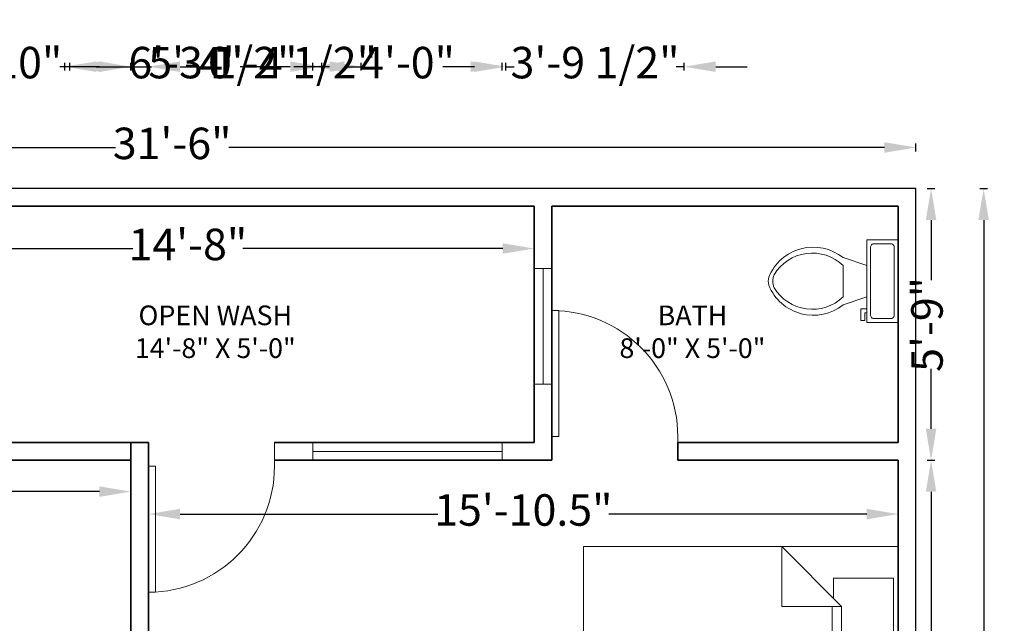
# Model space of a CAD drawing. Units: inches. Extents: x 2174 to 2692, y 577 to 1264.
# Tile 5 of 5: x 2442 to 2692, y 1110 to 1263. Entities that reach past the tile are written whole.
import ezdxf

# ---------------------------------------------------------------- set-up
doc = ezdxf.new("R2010")
doc.units = ezdxf.units.IN
for name, color, linetype, lineweight in [('A-ANNO-DIMS', 2, 'Continuous', 13), ('A-AREA-IDEN', 7, 'Continuous', 18), ('A-DOOR', 3, 'Continuous', 18), ('A-FLOR-FIXT', 9, 'Continuous', 18), ('A-FURN', 8, 'Continuous', 18), ('A-GLAZ', 4, 'Continuous', 18), ('A-WALL', 7, 'Continuous', 35), ('C-PROP', 7, 'Continuous', 25)]:
    doc.layers.add(name, color=color, linetype=linetype, lineweight=lineweight)
doc.styles.get("Standard").update_dxf_attribs({"font": 'arial.ttf'})
doc.dimstyles.new('ISO-25', dxfattribs={"dimtxt": 8, "dimasz": 8, "dimexe": 1, "dimexo": 1, "dimtad": 0, "dimdec": 1, "dimlunit": 3, "dimtxsty": 'Standard', "dimcen": 2.5, "dimclrd": 1, "dimclre": 1, "dimclrt": 1, "dimadec": 0, "dimazin": 0, "dimtfac": 1, "dimtdec": 1, "dimtmove": 0, "dimatfit": 3, "dimfxl": 1, "dimfxlon": 1, "dimarcsym": 0})

# ---------------------------------------------------------------- blocks, each defined once
blk = doc.blocks.new('Bed - Queen')
for p, q in [((0, -80.00003), (0, 0)), ((0, 0), (59.99999, 0)), ((59.99999, 0), (59.99999, -80.00003)), ((7.99999, -1.2), (28.79998, -1.2)), ((7.99999, -14.4), (7.99999, -1.2)), ((28.79998, -1.2), (28.79998, -14.4)), ((31.19999, -1.2), (51.99999, -1.2)), ((31.19999, -14.4), (31.19999, -1.2)), ((51.99999, -1.2), (51.99999, -16.4)), ((0, -14.4), (44.8, -14.4)), ((59.99999, -29.6), (44.8, -14.4)), ((44.8, -14.4), (44.8, -29.6)), ((44.8, -16.8), (0, -16.8)), ((51.99999, -16.4), (46.79936, -16.4)), ((44.8, -29.6), (59.99999, -29.6)), ((59.99999, -80.00003), (0, -80.00003))]:
    blk.add_line(p, q)
blk = doc.blocks.new('Toilet - top')
for p, q in [((9.5, -6), (9.5, -2)), ((-10, -8.5), (-8, -8.5)), ((-10, -9.5), (-10, -8.5)), ((-7, -9.5), (-10, -9.5)), ((-8, -8.5), (-8, -8)), ((-7, -8), (-7, -9.5)), ((-4, -8), (-6, -14)), ((4, -8), (6, -14)), ((4, -14), (-4, -14))]:
    blk.add_line(p, q)
blk.add_lwpolyline([(10.5, -8), (10.5, 0), (-10.5, 0), (-10.5, -8)], close=True)
for points in [[(-9.5, -2), (-9.5, -6)], [(8.5, -1), (-8.5, -1)], [(-8.5, -7), (8.5, -7)]]:
    blk.add_lwpolyline(points)
for centre, radius, start, end in [((-8.62, -1.88), 0.884, 81.8699, 188.1301), ((8.62, -1.88), 0.884, 351.8699, 98.1301), ((-8.62, -6.12), 0.884, 171.8699, 278.1301), ((8.62, -6.12), 0.884, 261.8699, 8.1301), ((3.52, -21.58), 12.17, 141.4691, 247.9714), ((4.2, -21.82), 11.33, 136.3677, 238.9468), ((-3.52, -21.58), 12.17, 292.0284, 38.5307), ((-4.2, -21.82), 11.33, 301.053, 43.6321), ((0, -27.88), 4, 245.7318, 294.2682), ((0, -29), 4, 254.8605, 285.1395)]:
    blk.add_arc(centre, radius, start, end)
blk = doc.blocks.new('*D9')
at = {"layer": 'A-ANNO-DIMS', "color": 0, "lineweight": -2, "transparency": 16777216}
for p, q in [((2396.95, 1206.12), (2396.95, 1204.12)), ((2572.95, 1206.12), (2572.95, 1204.12)), ((2404.95, 1205.12), (2470.96, 1205.12)), ((2564.95, 1205.12), (2498.94, 1205.12))]:
    blk.add_line(p, q, dxfattribs=at)
at = {"layer": 'A-ANNO-DIMS', "color": 0, "transparency": 16777216}
for points in [[(2404.95, 1206.46), (2404.95, 1203.79), (2396.95, 1205.12)], [(2564.95, 1206.46), (2564.95, 1203.79), (2572.95, 1205.12)]]:
    blk.add_solid(points, dxfattribs=at)
at = {"layer": 'Defpoints', "color": 0, "transparency": 16777216}
for p in [(2396.95, 1215.85), (2572.95, 1215.85), (2396.95, 1205.12)]:
    blk.add_point(p, dxfattribs=at)
at = {"layer": 'A-ANNO-DIMS', "color": 0, "transparency": 16777216, "insert": (2484.95, 1205.12), "char_height": 8, "attachment_point": 5}
blk.add_mtext('14\'-8"', dxfattribs=at)
blk = doc.blocks.new('*D10')
at = {"layer": 'A-ANNO-DIMS', "color": 0, "lineweight": -2, "transparency": 16777216}
for p, q in [((2665.45, 1137.68), (2665.45, 1138.68)), ((2474.95, 1137.68), (2474.95, 1136.68)), ((2482.95, 1137.68), (2548.45, 1137.68)), ((2657.45, 1137.68), (2591.96, 1137.68))]:
    blk.add_line(p, q, dxfattribs=at)
at = {"layer": 'A-ANNO-DIMS', "color": 0, "transparency": 16777216}
for points in [[(2482.95, 1139.02), (2482.95, 1136.35), (2474.95, 1137.68)], [(2657.45, 1139.02), (2657.45, 1136.35), (2665.45, 1137.68)]]:
    blk.add_solid(points, dxfattribs=at)
at = {"layer": 'Defpoints', "color": 0, "transparency": 16777216}
for p in [(2474.95, 1137.68), (2665.45, 1137.68), (2665.45, 1137.68)]:
    blk.add_point(p, dxfattribs=at)
at = {"layer": 'A-ANNO-DIMS', "color": 0, "transparency": 16777216, "insert": (2570.2, 1137.68), "char_height": 8, "attachment_point": 5}
blk.add_mtext('15\'-10.5"', dxfattribs=at)
blk = doc.blocks.new('*D11')
at = {"layer": 'A-ANNO-DIMS', "color": 0, "lineweight": -2, "transparency": 16777216}
for p, q in [((2296.45, 1144.39), (2296.45, 1142.39)), ((2470.45, 1144.39), (2470.45, 1142.39)), ((2304.45, 1143.39), (2369.46, 1143.39)), ((2462.45, 1143.39), (2397.44, 1143.39))]:
    blk.add_line(p, q, dxfattribs=at)
at = {"layer": 'A-ANNO-DIMS', "color": 0, "transparency": 16777216}
for points in [[(2304.45, 1144.72), (2304.45, 1142.05), (2296.45, 1143.39)], [(2462.45, 1144.72), (2462.45, 1142.05), (2470.45, 1143.39)]]:
    blk.add_solid(points, dxfattribs=at)
at = {"layer": 'Defpoints', "color": 0, "transparency": 16777216}
for p in [(2296.45, 1151.35), (2470.45, 1151.35), (2470.45, 1143.39)]:
    blk.add_point(p, dxfattribs=at)
at = {"layer": 'A-ANNO-DIMS', "color": 0, "transparency": 16777216, "insert": (2383.45, 1143.39), "char_height": 8, "attachment_point": 5}
blk.add_mtext('14\'-6"', dxfattribs=at)
blk = doc.blocks.new('*U23')
for p, q in [((0, 0), (0, 6)), ((32, 0), (32, 6))]:
    blk.add_line(p, q)
blk.add_lwpolyline([(0, 0), (0, -32), (1.75, -32), (1.75, 0)], close=True)
blk.add_arc((0, 0), 32, 270, 0)
blk = doc.blocks.new('*U22')
for p, q in [((0, 0), (0, -6)), ((32, 0), (32, -6))]:
    blk.add_line(p, q)
blk.add_lwpolyline([(0, 0), (0, 32), (1.75, 32), (1.75, 0)], close=True)
blk.add_arc((0, 0), 32, 0, 90)
blk = doc.blocks.new('*D28')
at = {"layer": 'A-ANNO-DIMS', "color": 0, "lineweight": -2, "transparency": 16777216}
for p, q in [((2291.95, 1229.78), (2291.95, 1231.78)), ((2669.95, 1229.78), (2669.95, 1231.78)), ((2299.95, 1230.78), (2466.59, 1230.78)), ((2661.95, 1230.78), (2495.32, 1230.78))]:
    blk.add_line(p, q, dxfattribs=at)
at = {"layer": 'A-ANNO-DIMS', "color": 0, "transparency": 16777216}
for points in [[(2299.95, 1232.11), (2299.95, 1229.44), (2291.95, 1230.78)], [(2661.95, 1232.11), (2661.95, 1229.44), (2669.95, 1230.78)]]:
    blk.add_solid(points, dxfattribs=at)
at = {"layer": 'Defpoints', "color": 0, "transparency": 16777216}
for p in [(2669.95, 1230.78), (2291.95, 1220.35), (2669.95, 1220.35)]:
    blk.add_point(p, dxfattribs=at)
at = {"layer": 'A-ANNO-DIMS', "color": 0, "transparency": 16777216, "insert": (2480.95, 1230.78), "char_height": 8, "attachment_point": 5}
blk.add_mtext('31\'-6"', dxfattribs=at)
blk = doc.blocks.new('*D35')
at = {"layer": 'A-ANNO-DIMS', "color": 0, "lineweight": -2, "transparency": 16777216}
for p, q in [((2672.81, 1220.35), (2674.81, 1220.35)), ((2673.81, 1212.35), (2673.81, 1197.11)), ((2673.81, 1159.35), (2673.81, 1174.59)), ((2672.81, 1151.35), (2674.81, 1151.35))]:
    blk.add_line(p, q, dxfattribs=at)
at = {"layer": 'A-ANNO-DIMS', "color": 0, "transparency": 16777216}
for points in [[(2672.48, 1212.35), (2675.15, 1212.35), (2673.81, 1220.35)], [(2672.48, 1159.35), (2675.15, 1159.35), (2673.81, 1151.35)]]:
    blk.add_solid(points, dxfattribs=at)
at = {"layer": 'Defpoints', "color": 0, "transparency": 16777216}
for p in [(2669.95, 1220.35), (2665.45, 1151.35), (2673.81, 1151.35)]:
    blk.add_point(p, dxfattribs=at)
at = {"layer": 'A-ANNO-DIMS', "color": 0, "transparency": 16777216, "insert": (2673.81, 1185.85), "char_height": 8, "attachment_point": 5, "rotation": 90}
blk.add_mtext('5\'-9"', dxfattribs=at)
blk = doc.blocks.new('*D36')
at = {"layer": 'A-ANNO-DIMS', "color": 0, "lineweight": -2, "transparency": 16777216}
for p, q in [((2672.81, 1151.35), (2674.81, 1151.35)), ((2673.81, 1143.35), (2673.81, 1101.75)), ((2673.81, 1022.85), (2673.81, 1064.45)), ((2672.81, 1014.85), (2674.81, 1014.85))]:
    blk.add_line(p, q, dxfattribs=at)
at = {"layer": 'A-ANNO-DIMS', "color": 0, "transparency": 16777216}
for points in [[(2672.48, 1143.35), (2675.15, 1143.35), (2673.81, 1151.35)], [(2672.48, 1022.85), (2675.15, 1022.85), (2673.81, 1014.85)]]:
    blk.add_solid(points, dxfattribs=at)
at = {"layer": 'Defpoints', "color": 0, "transparency": 16777216}
for p in [(2665.45, 1151.35), (2665.45, 1014.85), (2673.81, 1014.85)]:
    blk.add_point(p, dxfattribs=at)
at = {"layer": 'A-ANNO-DIMS', "color": 0, "transparency": 16777216, "insert": (2673.81, 1083.1), "char_height": 8, "attachment_point": 5, "rotation": 90}
blk.add_mtext('11\'-4.5"', dxfattribs=at)
blk = doc.blocks.new('*D42')
at = {"layer": 'A-ANNO-DIMS', "color": 0, "lineweight": -2, "transparency": 16777216}
for p, q in [((2686.18, 1220.35), (2688.18, 1220.35)), ((2687.18, 1212.35), (2687.18, 927.77)), ((2687.18, 628.35), (2687.18, 912.94)), ((2686.18, 620.35), (2688.18, 620.35))]:
    blk.add_line(p, q, dxfattribs=at)
at = {"layer": 'A-ANNO-DIMS', "color": 0, "transparency": 16777216}
for points in [[(2685.84, 1212.35), (2688.51, 1212.35), (2687.18, 1220.35)], [(2685.84, 628.35), (2688.51, 628.35), (2687.18, 620.35)]]:
    blk.add_solid(points, dxfattribs=at)
at = {"layer": 'Defpoints', "color": 0, "transparency": 16777216}
for p in [(2669.95, 1220.35), (2687.18, 1220.35), (2669.95, 620.35)]:
    blk.add_point(p, dxfattribs=at)
at = {"layer": 'A-ANNO-DIMS', "color": 0, "transparency": 16777216, "insert": (2687.18, 920.35), "char_height": 8, "attachment_point": 5, "rotation": 90}
blk.add_mtext("50'", dxfattribs=at)
blk = doc.blocks.new('*D65')
at = {"layer": 'A-ANNO-DIMS', "color": 1, "lineweight": -2, "transparency": 16777216}
for p, q in [((2412.95, 1251.3), (2404.95, 1251.3)), ((2420.95, 1250.3), (2420.95, 1252.3)), ((2420.95, 1251.3), (2423.52, 1251.3)), ((2454.95, 1251.3), (2452.39, 1251.3)), ((2454.95, 1250.3), (2454.95, 1252.3)), ((2462.95, 1251.3), (2470.95, 1251.3))]:
    blk.add_line(p, q, dxfattribs=at)
at = {"layer": 'A-ANNO-DIMS', "color": 1, "transparency": 16777216}
for points in [[(2412.95, 1252.64), (2412.95, 1249.97), (2420.95, 1251.3)], [(2462.95, 1252.64), (2462.95, 1249.97), (2454.95, 1251.3)]]:
    blk.add_solid(points, dxfattribs=at)
at = {"layer": 'Defpoints', "color": 0, "transparency": 16777216}
for p in [(2454.95, 1251.3), (2420.95, 698.35), (2454.95, 698.35)]:
    blk.add_point(p, dxfattribs=at)
at = {"layer": 'A-ANNO-DIMS', "color": 1, "transparency": 16777216, "insert": (2437.95, 1251.3), "char_height": 8, "attachment_point": 5}
blk.add_mtext('2\'-10"', dxfattribs=at)
blk = doc.blocks.new('*D66')
at = {"layer": 'A-ANNO-DIMS', "color": 1, "lineweight": -2, "transparency": 16777216}
for p, q in [((2454.95, 1250.3), (2454.95, 1252.3)), ((2462.95, 1251.3), (2475.7, 1251.3)), ((2510.95, 1251.3), (2498.21, 1251.3)), ((2518.95, 1250.3), (2518.95, 1252.3))]:
    blk.add_line(p, q, dxfattribs=at)
at = {"layer": 'A-ANNO-DIMS', "color": 1, "transparency": 16777216}
for points in [[(2462.95, 1252.64), (2462.95, 1249.97), (2454.95, 1251.3)], [(2510.95, 1252.64), (2510.95, 1249.97), (2518.95, 1251.3)]]:
    blk.add_solid(points, dxfattribs=at)
at = {"layer": 'Defpoints', "color": 0, "transparency": 16777216}
for p in [(2518.95, 1251.3), (2454.95, 698.35), (2518.95, 698.35)]:
    blk.add_point(p, dxfattribs=at)
at = {"layer": 'A-ANNO-DIMS', "color": 1, "transparency": 16777216, "insert": (2486.95, 1251.3), "char_height": 8, "attachment_point": 5}
blk.add_mtext('5\'-4"', dxfattribs=at)
blk = doc.blocks.new('*D69')
at = {"layer": 'A-ANNO-DIMS', "color": 1, "lineweight": -2, "transparency": 16777216}
for p, q in [((2453.65, 1250.3), (2453.65, 1252.3)), ((2461.65, 1251.3), (2470.7, 1251.3)), ((2520.95, 1251.3), (2511.9, 1251.3)), ((2528.95, 1250.3), (2528.95, 1252.3))]:
    blk.add_line(p, q, dxfattribs=at)
at = {"layer": 'A-ANNO-DIMS', "color": 1, "transparency": 16777216}
for points in [[(2461.65, 1252.64), (2461.65, 1249.97), (2453.65, 1251.3)], [(2520.95, 1252.64), (2520.95, 1249.97), (2528.95, 1251.3)]]:
    blk.add_solid(points, dxfattribs=at)
at = {"layer": 'Defpoints', "color": 0, "transparency": 16777216}
for p in [(2528.95, 1251.3), (2453.65, 878.35), (2528.95, 878.35)]:
    blk.add_point(p, dxfattribs=at)
at = {"layer": 'A-ANNO-DIMS', "color": 1, "transparency": 16777216, "insert": (2491.3, 1251.3), "char_height": 8, "attachment_point": 5}
blk.add_mtext('6\'-3 1/2"', dxfattribs=at)
blk = doc.blocks.new('*D74')
at = {"layer": 'A-ANNO-DIMS', "color": 1, "lineweight": -2, "transparency": 16777216}
for p, q in [((2557.76, 1251.3), (2549.76, 1251.3)), ((2565.76, 1250.3), (2565.76, 1252.3)), ((2565.76, 1251.3), (2567.84, 1251.3)), ((2611.08, 1251.3), (2609, 1251.3)), ((2611.08, 1250.3), (2611.08, 1252.3)), ((2619.08, 1251.3), (2627.08, 1251.3))]:
    blk.add_line(p, q, dxfattribs=at)
at = {"layer": 'A-ANNO-DIMS', "color": 1, "transparency": 16777216}
for points in [[(2557.76, 1252.64), (2557.76, 1249.97), (2565.76, 1251.3)], [(2619.08, 1252.64), (2619.08, 1249.97), (2611.08, 1251.3)]]:
    blk.add_solid(points, dxfattribs=at)
at = {"layer": 'Defpoints', "color": 0, "transparency": 16777216}
for p in [(2611.08, 1251.3), (2565.76, 882.85), (2611.08, 882.85)]:
    blk.add_point(p, dxfattribs=at)
at = {"layer": 'A-ANNO-DIMS', "color": 1, "transparency": 16777216, "insert": (2588.42, 1251.3), "char_height": 8, "attachment_point": 5}
blk.add_mtext('3\'-9 1/2"', dxfattribs=at)
blk = doc.blocks.new('*D76')
at = {"layer": 'A-ANNO-DIMS', "color": 1, "lineweight": -2, "transparency": 16777216}
for p, q in [((2462.45, 1251.3), (2454.45, 1251.3)), ((2470.45, 1250.3), (2470.45, 1252.3)), ((2470.45, 1251.3), (2474.95, 1251.3)), ((2474.95, 1250.3), (2474.95, 1252.3)), ((2482.95, 1251.3), (2490.95, 1251.3))]:
    blk.add_line(p, q, dxfattribs=at)
at = {"layer": 'A-ANNO-DIMS', "color": 1, "transparency": 16777216}
for points in [[(2462.45, 1252.64), (2462.45, 1249.97), (2470.45, 1251.3)], [(2482.95, 1252.64), (2482.95, 1249.97), (2474.95, 1251.3)]]:
    blk.add_solid(points, dxfattribs=at)
at = {"layer": 'Defpoints', "color": 0, "transparency": 16777216}
for p in [(2474.95, 1251.3), (2470.45, 1151.35), (2474.95, 1151.6)]:
    blk.add_point(p, dxfattribs=at)
at = {"layer": 'A-ANNO-DIMS', "color": 1, "transparency": 16777216, "insert": (2511.53, 1251.3), "char_height": 8, "attachment_point": 5}
blk.add_mtext('0\'-4 1/2"', dxfattribs=at)
blk = doc.blocks.new('*D78')
at = {"layer": 'A-ANNO-DIMS', "color": 1, "lineweight": -2, "transparency": 16777216}
for p, q in [((2399.49, 590.4), (2399.49, 588.4)), ((2407.49, 589.4), (2424.76, 589.4)), ((2432.76, 590.4), (2432.76, 588.4)), ((2432.76, 589.4), (2440.76, 589.4))]:
    blk.add_line(p, q, dxfattribs=at)
at = {"layer": 'A-ANNO-DIMS', "color": 1, "transparency": 16777216}
for points in [[(2407.49, 590.74), (2407.49, 588.07), (2399.49, 589.4)], [(2424.76, 590.74), (2424.76, 588.07), (2432.76, 589.4)]]:
    blk.add_solid(points, dxfattribs=at)
at = {"layer": 'Defpoints', "color": 0, "transparency": 16777216}
for p in [(2399.49, 1151.35), (2432.76, 1151.35), (2432.76, 589.4)]:
    blk.add_point(p, dxfattribs=at)
at = {"layer": 'A-ANNO-DIMS', "color": 1, "transparency": 16777216, "insert": (2461.41, 589.4), "char_height": 8, "attachment_point": 5}
blk.add_mtext('2\'-9 1/2"', dxfattribs=at)
blk = doc.blocks.new('*D79')
at = {"layer": 'A-ANNO-DIMS', "color": 1, "lineweight": -2, "transparency": 16777216}
for p, q in [((2516.7, 1250.3), (2516.7, 1252.3)), ((2524.7, 1251.3), (2529.35, 1251.3)), ((2556.84, 1251.3), (2552.18, 1251.3)), ((2564.84, 1250.3), (2564.84, 1252.3))]:
    blk.add_line(p, q, dxfattribs=at)
at = {"layer": 'A-ANNO-DIMS', "color": 1, "transparency": 16777216}
for points in [[(2524.7, 1252.64), (2524.7, 1249.97), (2516.7, 1251.3)], [(2556.84, 1252.64), (2556.84, 1249.97), (2564.84, 1251.3)]]:
    blk.add_solid(points, dxfattribs=at)
at = {"layer": 'Defpoints', "color": 0, "transparency": 16777216}
for p in [(2564.84, 1251.3), (2516.7, 1155.85), (2564.84, 1155.85)]:
    blk.add_point(p, dxfattribs=at)
at = {"layer": 'A-ANNO-DIMS', "color": 1, "transparency": 16777216, "insert": (2540.77, 1251.3), "char_height": 8, "attachment_point": 5}
blk.add_mtext('4\'-0"', dxfattribs=at)
blk = doc.blocks.new('*D80')
at = {"layer": 'A-ANNO-DIMS', "color": 1, "lineweight": -2, "transparency": 16777216}
for p, q in [((2577.45, 590.4), (2577.45, 588.4)), ((2585.45, 589.4), (2610.23, 589.4)), ((2657.45, 589.4), (2632.68, 589.4)), ((2665.45, 590.4), (2665.45, 588.4))]:
    blk.add_line(p, q, dxfattribs=at)
at = {"layer": 'A-ANNO-DIMS', "color": 1, "transparency": 16777216}
for points in [[(2585.45, 590.74), (2585.45, 588.07), (2577.45, 589.4)], [(2657.45, 590.74), (2657.45, 588.07), (2665.45, 589.4)]]:
    blk.add_solid(points, dxfattribs=at)
at = {"layer": 'Defpoints', "color": 0, "transparency": 16777216}
for p in [(2577.45, 1215.85), (2665.45, 1215.85), (2665.45, 589.4)]:
    blk.add_point(p, dxfattribs=at)
at = {"layer": 'A-ANNO-DIMS', "color": 1, "transparency": 16777216, "insert": (2621.45, 589.4), "char_height": 8, "attachment_point": 5}
blk.add_mtext('7\'-4"', dxfattribs=at)

msp = doc.modelspace()

# ---------------------------------------------------------------- linework, layer by layer
at = {"layer": 'A-GLAZ'}
for p, q in [((2572.95, 1200.08), (2577.45, 1200.08)), ((2575.2, 1170.69), (2575.2, 1200.08)), ((2572.95, 1170.69), (2577.45, 1170.69)), ((2516.7, 1155.85), (2516.7, 1151.35)), ((2516.7, 1153.6), (2564.84, 1153.6)), ((2564.84, 1155.85), (2564.84, 1151.35))]:
    msp.add_line(p, q, dxfattribs=at)
at = {"layer": 'A-WALL'}
for p, q in [((2572.95, 1215.85), (2396.95, 1215.85)), ((2572.95, 1215.85), (2572.95, 1155.85)), ((2665.45, 1215.85), (2577.45, 1215.85)), ((2577.45, 1215.85), (2577.45, 1155.85)), ((2665.45, 1155.85), (2665.45, 1215.85)), ((2470.45, 1155.85), (2396.95, 1155.85)), ((2470.45, 1155.85), (2470.45, 1023.85)), ((2474.95, 1155.85), (2470.45, 1155.85)), ((2474.95, 1155.85), (2474.95, 1019.35)), ((2572.95, 1155.85), (2506.95, 1155.85)), ((2577.45, 1155.85), (2577.45, 1151.35)), ((2665.45, 1155.85), (2609.45, 1155.85)), ((2609.45, 1155.85), (2609.45, 1151.35)), ((2470.45, 1151.35), (2392.45, 1151.35)), ((2577.45, 1151.35), (2506.95, 1151.35)), ((2665.45, 1151.35), (2609.45, 1151.35)), ((2665.45, 1019.35), (2665.45, 1151.35))]:
    msp.add_line(p, q, dxfattribs=at)
at = {"layer": 'C-PROP'}
for p, q in [((2669.95, 1220.35), (2291.95, 1220.35)), ((2669.95, 620.35), (2669.95, 1220.35))]:
    msp.add_line(p, q, dxfattribs=at)

# ---------------------------------------------------------------- block references
at = {"layer": 'A-DOOR'}
for name, p in [('*U22', (2577.45, 1157.35)), ('*U23', (2474.95, 1149.85))]:
    msp.add_blockref(name, p, dxfattribs=at)
at = {"layer": 'A-FLOR-FIXT', "xscale": -1, "rotation": 270}
msp.add_blockref('Toilet - top', (2665.45, 1196.82), dxfattribs=at)
at = {"layer": 'A-FURN', "xscale": -1, "rotation": 269.9999999999765}
msp.add_blockref('Bed - Queen', (2665.45, 1069.43), dxfattribs=at)

# ---------------------------------------------------------------- texts
at = {"layer": 'A-AREA-IDEN', "char_height": 5, "attachment_point": 1}
for s, width, insert in [('\\pxqc;OPEN WASH\\P14\'-8" X 5\'-0"', 50.1555, (2466.83, 1190.65)), ('\\pxqc;BATH\\P8\'-0" X 5\'-0"', 38.1431, (2594.1, 1190.65))]:
    msp.add_mtext_dynamic_manual_height_columns(s, width=width, gutter_width=12.5, heights=[0], dxfattribs=dict(at, insert=insert))

# ---------------------------------------------------------------- dimensions: what is measured, and where the dimension line sits
at = {"layer": 'A-ANNO-DIMS'}
for base, p1, p2, override, picture, middle in [((2528.95, 1251.3), (2453.65, 878.35), (2528.95, 878.35), {"dimdec": 1, "dimlfac": 1, "dimrnd": 0, "dimzin": 1, "dimdsep": 46, "dimlunit": 4, "dimfrac": 2}, '*D69', (2491.3, 1251.3)), ((2474.95, 1251.3), (2470.45, 1151.35), (2474.95, 1151.6), {"dimdec": 1, "dimlfac": 1, "dimrnd": 0, "dimzin": 1, "dimdsep": 46, "dimlunit": 4, "dimfrac": 2}, '*D76', (2511.53, 1251.3)), ((2611.08, 1251.3), (2565.76, 882.85), (2611.08, 882.85), {"dimdec": 1, "dimlfac": 1, "dimrnd": 0, "dimzin": 1, "dimdsep": 46, "dimlunit": 4, "dimfrac": 2}, '*D74', (2588.42, 1251.3)), ((2454.95, 1251.3), (2420.95, 698.35), (2454.95, 698.35), {"dimdec": 1, "dimlfac": 1, "dimrnd": 0, "dimzin": 1, "dimdsep": 46, "dimlunit": 4, "dimfrac": 2}, '*D65', (2437.95, 1251.3)), ((2518.95, 1251.3), (2454.95, 698.35), (2518.95, 698.35), {"dimdec": 1, "dimlfac": 1, "dimrnd": 0, "dimzin": 1, "dimdsep": 46, "dimlunit": 4, "dimfrac": 2}, '*D66', (2486.95, 1251.3)), ((2564.84, 1251.3), (2516.7, 1155.85), (2564.84, 1155.85), {"dimdec": 1, "dimlfac": 1, "dimrnd": 0, "dimzin": 1, "dimdsep": 46, "dimlunit": 4, "dimfrac": 2}, '*D79', (2540.77, 1251.3)), ((2669.95, 1230.78), (2291.95, 1220.35), (2669.95, 1220.35), {"dimclrd": 0, "dimclre": 0, "dimclrt": 0}, '*D28', (2480.95, 1230.78)), ((2396.95, 1205.12), (2572.95, 1215.85), (2396.95, 1215.85), {"dimclrd": 0, "dimclre": 0, "dimclrt": 0}, '*D9', (2484.95, 1205.12)), ((2665.45, 589.4), (2577.45, 1215.85), (2665.45, 1215.85), {"dimdec": 1, "dimlfac": 1, "dimrnd": 0, "dimzin": 1, "dimdsep": 46, "dimlunit": 4, "dimfrac": 2}, '*D80', (2621.45, 589.4)), ((2432.76, 589.4), (2399.49, 1151.35), (2432.76, 1151.35), {"dimdec": 1, "dimlfac": 1, "dimrnd": 0, "dimzin": 1, "dimdsep": 46, "dimlunit": 4, "dimfrac": 2}, '*D78', (2461.41, 589.4)), ((2665.45, 1137.68), (2474.95, 1137.68), (2665.45, 1137.68), {"dimclrd": 0, "dimclre": 0, "dimclrt": 0}, '*D10', (2570.2, 1137.68))]:
    dim = msp.add_linear_dim(base=base, p1=p1, p2=p2, dimstyle='ISO-25', override=override, dxfattribs=at)
    dim.commit()
    dim.dimension.update_dxf_attribs({"geometry": picture, "text_midpoint": middle})
for base, p1, p2, override, picture, middle in [((2673.81, 1151.35), (2669.95, 1220.35), (2665.45, 1151.35), {"dimclrd": 0, "dimclre": 0, "dimclrt": 0}, '*D35', (2673.81, 1185.85)), ((2687.18, 1220.35), (2669.95, 620.35), (2669.95, 1220.35), {"dimclrd": 0, "dimclre": 0, "dimclrt": 0}, '*D42', (2687.18, 920.35)), ((2673.81, 1014.85), (2665.45, 1151.35), (2665.45, 1014.85), {"dimclrd": 0, "dimclre": 0, "dimclrt": 0, "dimtmove": 1}, '*D36', (2673.81, 1083.1))]:
    dim = msp.add_linear_dim(base=base, p1=p1, p2=p2, angle=90, dimstyle='ISO-25', override=override, dxfattribs=at)
    dim.commit()
    dim.dimension.update_dxf_attribs({"geometry": picture, "text_midpoint": middle})
dim = msp.add_linear_dim(base=(2470.45, 1143.39), p1=(2296.45, 1151.35), p2=(2470.45, 1151.35), dimstyle='ISO-25', override={"dimclrd": 0, "dimclre": 0, "dimclrt": 0}, dxfattribs=at)
dim.commit()
dim.dimension.update_dxf_attribs({"geometry": '*D11', "text_midpoint": (2383.45, 1143.39), "dimtype": 160})

doc.saveas('drawing.dxf')
